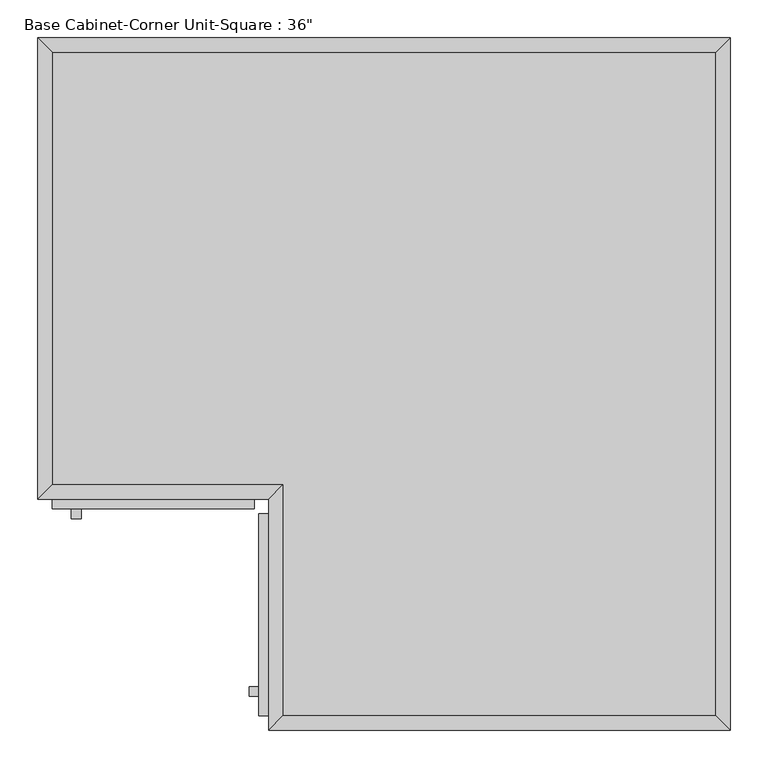
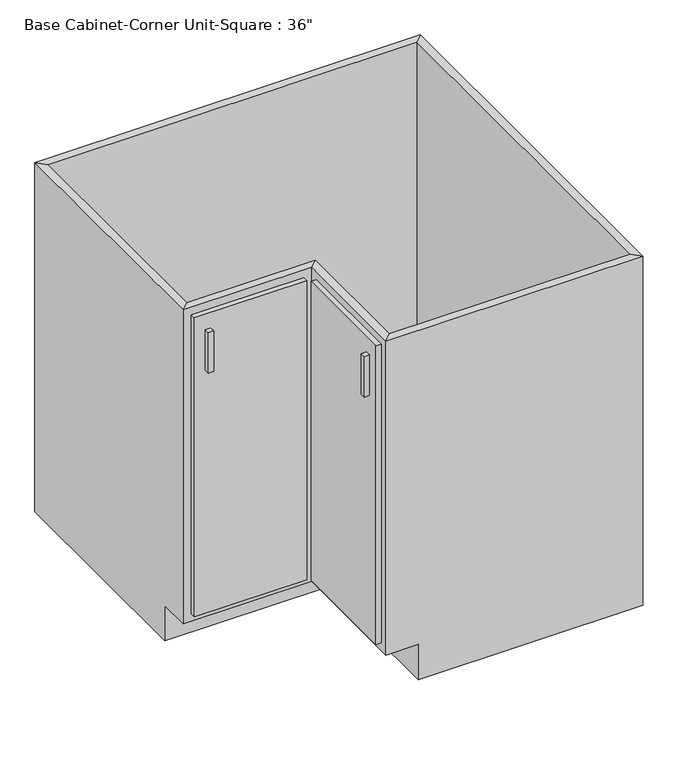
"""IFC4 building model written with IfcOpenShell, lengths in millimetres: furniture geometry."""

from ifc_helpers import new_model, si_unit, frame, origin, place, context, project, spatial, polyline, outline, extrude, faceted_brep, source, transform, mapped, element, save


def furniture_97fe820d(model_context):
    return source(origin(), model_context, "Body", "SolidModel", [
        extrude(outline(polyline([(507.6877049, -19.05), (507.6877049, -895.35), (-63.8122951, -895.35), (-63.8122951, -590.55), (-368.6122951, -590.55), (-368.6122951, -19.05), (507.6877049, -19.05)])), frame((0.0, 0.0, 88.9), z_axis=(0.0, 0.0, 1.0), x_axis=(1.0, 0.0, 0.0)), (0.0, 0.0, 1.0), 19.05),
        extrude(outline(polyline([(-101.9122951, -622.3), (-368.6122951, -622.3), (-368.6122951, -609.6), (-101.9122951, -609.6), (-101.9122951, -622.3)])), frame((0.0, 0.0, 107.95), z_axis=(0.0, 0.0, 1.0), x_axis=(1.0, 0.0, 0.0)), (0.0, 0.0, 1.0), 749.3),
        extrude(outline(polyline([(-330.5122951, -635.0), (-343.2122951, -635.0), (-343.2122951, -622.3), (-330.5122951, -622.3), (-330.5122951, -635.0)])), frame((0.0, 0.0, 717.55), z_axis=(0.0, 0.0, 1.0), x_axis=(1.0, 0.0, 0.0)), (0.0, 0.0, 1.0), 101.6),
        extrude(outline(polyline([(-82.8622951, -628.65), (-82.8622951, -895.35), (-95.5622951, -895.35), (-95.5622951, -628.65), (-82.8622951, -628.65)])), frame((0.0, 0.0, 107.95), z_axis=(0.0, 0.0, 1.0), x_axis=(1.0, 0.0, 0.0)), (0.0, 0.0, 1.0), 749.3),
        extrude(outline(polyline([(-95.5622951, -857.25), (-95.5622951, -869.95), (-108.2622951, -869.95), (-108.2622951, -857.25), (-95.5622951, -857.25)])), frame((0.0, 0.0, 717.55), z_axis=(0.0, 0.0, 1.0), x_axis=(1.0, 0.0, 0.0)), (0.0, 0.0, 1.0), 101.6),
        faceted_brep([(-368.6122951, -533.4, 88.9), (-6.6622951, -533.4, 88.9), (-6.6622951, -895.35, 88.9), (507.6877049, -895.35, 88.9), (507.6877049, -19.05, 88.9), (-368.6122951, -19.05, 88.9), (526.7377049, 0.0, 0.0), (526.7377049, -914.4, 0.0), (-6.6622951, -914.4, 0.0), (-6.6622951, -533.4, 0.0), (-387.6622951, -533.4, 0.0), (-387.6622951, 0.0, 0.0), (-387.6622951, 0.0, 876.3), (526.7377049, 0.0, 876.3), (-387.6622951, -533.4, 88.9), (-387.6622951, -609.6, 88.9), (-387.6622951, -609.6, 876.3), (-6.6622951, -914.4, 88.9), (526.7377049, -914.4, 876.3), (-82.8622951, -914.4, 876.3), (-82.8622951, -914.4, 88.9), (507.6877049, -895.35, 876.3), (-63.8122951, -895.35, 88.9), (-63.8122951, -895.35, 876.3), (-63.8122951, -590.55, 88.9), (-63.8122951, -590.55, 876.3), (-82.8622951, -609.6, 876.3), (-82.8622951, -609.6, 88.9), (-368.6122951, -590.55, 88.9), (-368.6122951, -590.55, 876.3), (-368.6122951, -19.05, 876.3), (507.6877049, -19.05, 876.3)], [[[0, 1, 2, 3, 4, 5]], [[6, 7, 8, 9, 10, 11]], [[6, 11, 12, 13]], [[12, 11, 10, 14, 15, 16]], [[10, 9, 1, 0, 14]], [[9, 8, 17, 2, 1]], [[8, 7, 18, 19, 20, 17]], [[18, 7, 6, 13]], [[21, 3, 2, 22, 23]], [[21, 23, 19, 18]], [[20, 22, 2, 17]], [[23, 22, 24, 25]], [[19, 23, 25, 26]], [[20, 19, 26, 27]], [[22, 20, 27, 24]], [[25, 24, 28, 29]], [[26, 25, 29, 16]], [[27, 26, 16, 15]], [[24, 27, 15, 28]], [[29, 28, 0, 5, 30]], [[16, 29, 30, 12]], [[28, 15, 14, 0]], [[30, 5, 4, 31]], [[12, 30, 31, 13]], [[3, 21, 31, 4]], [[21, 18, 13, 31]]]),
    ])


if __name__ == "__main__":
    model = new_model("IFC4")
    model_context = context("Model", 3, world=origin())
    ifc_project = project(units=[si_unit("LENGTHUNIT", "METRE", prefix="MILLI")], contexts=[model_context])
    site = spatial("IfcSite", under=ifc_project)
    building = spatial("IfcBuilding", under=site)
    placement = place(None, origin())
    furniture_shape = furniture_97fe820d(model_context)
    element("IfcFurniture", 1, ObjectType="Base Cabinet-Corner Unit-Square : 36\"", at=placement, inside=building, context=model_context, shape_type="MappedRepresentation", body=[
        mapped(furniture_shape, transform((0.0, 0.0, 0.0), x_axis=(1.0, 0.0, 0.0), y_axis=(0.0, 1.0, 0.0), z_axis=(0.0, 0.0, 1.0))),
    ])
    save(model, "model.ifc")

# Revit data of these elements
# Type "Base Cabinet-Corner Unit-Square : 36\""
#   Assembly Code = "C1030410"
#   Depth = 2' - 0"
#   Height = 2' - 10 1/2"
#   Toe Depth = 0' - 3"
#   Toe Height = 0' - 3 1/2"
#   Width = 3' - 0"
#   Cabinet Material = Cabinets
#   Door/Drawer Material = Cabinets
#   Handle Material = Cabinets - Handles
#   Default Elevation = 0
# Element 1 (IfcFurniture, "Base Cabinet-Corner Unit-Square : 36\"")
#   Materials on its faces: "Cabinets", "Cabinets - Handles"
# Materials
#   "Cabinets": colour RGB 249 249 249, transparency 0
#   "Cabinets - Handles": class "Metal", colour RGB 57 57 57, transparency 0
